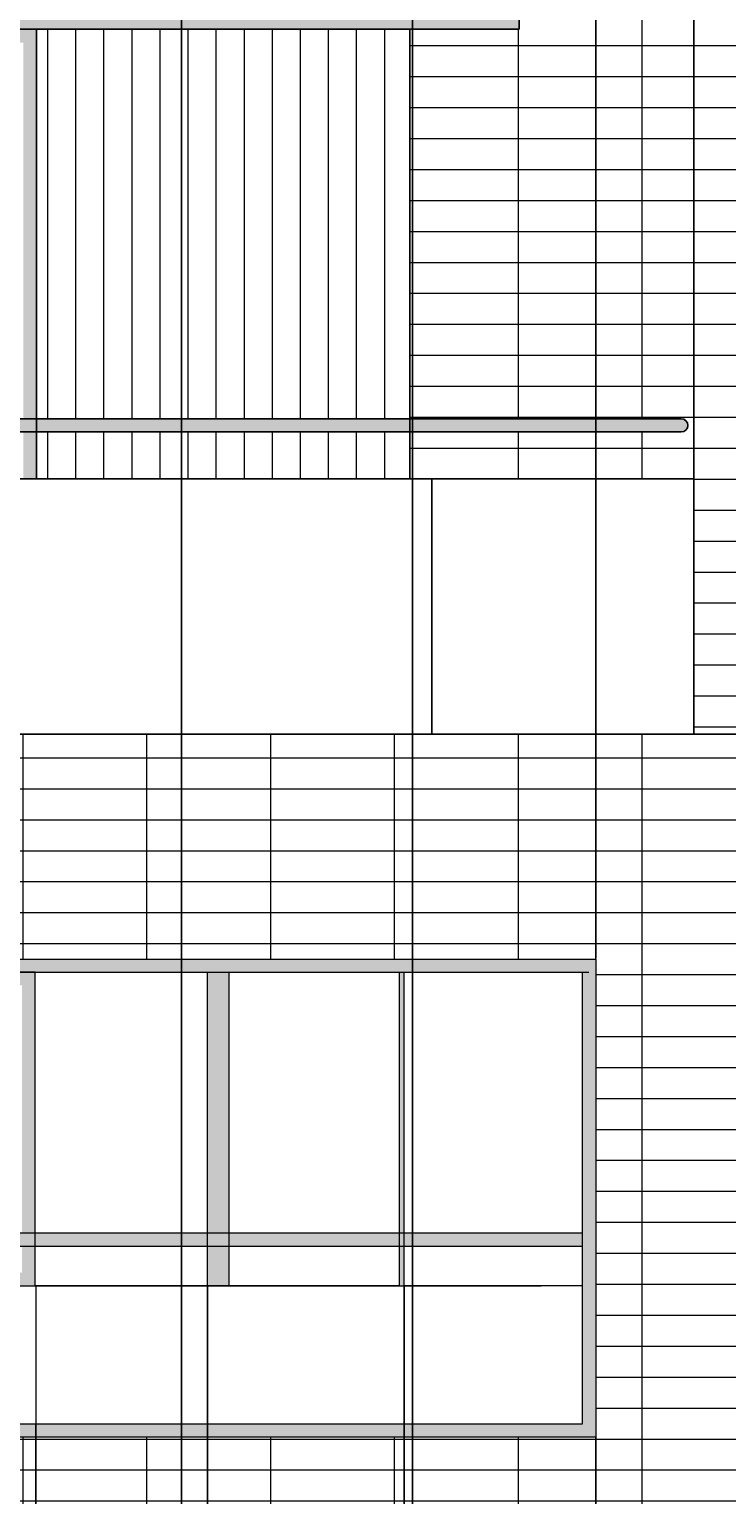
# Model space of a CAD drawing. Units: inches. Extents: x 241 to 943, y 109 to 1396.
# Tile 12 of 34: x 507 to 613, y 620 to 842. Entities that reach past the tile are written whole.
import ezdxf

# ---------------------------------------------------------------- set-up
doc = ezdxf.new("R2010")
doc.units = ezdxf.units.IN
doc.header["$MEASUREMENT"] = 0
for name, color, linetype, lineweight in [('A-ANNO-DIMS', 2, 'Continuous', 18), ('A-ELEV', 7, 'Continuous', 25), ('A-ELEV-SHAD', 9, 'Continuous', 13), ('A-GLAZ', 4, 'Continuous', 18), ('A-GLAZ-PATT', 18, 'Continuous', 13), ('A-WALL-PATT', 8, 'Continuous', 13)]:
    doc.layers.add(name, color=color, linetype=linetype, lineweight=lineweight)
doc.styles.get("Standard").update_dxf_attribs({"font": 'arial.ttf'})
doc.dimstyles.get("Standard").update_dxf_attribs({"dimtxt": 1.4375, "dimasz": 0.18, "dimexe": 0.18, "dimexo": 0.0625, "dimgap": 0.09, "dimtad": 0, "dimtih": 1, "dimtoh": 1, "dimdec": 4, "dimzin": 0, "dimdsep": 46, "dimlunit": 4, "dimtxsty": 'Standard', "dimcen": 0.09, "dimadec": 0, "dimazin": 0, "dimtfac": 1, "dimtdec": 4, "dimtofl": 0, "dimtmove": 0, "dimatfit": 3, "dimfxl": 1, "dimtolj": 1, "dimtzin": 0, "dimarcsym": 0})

# ---------------------------------------------------------------- blocks, each defined once
blk = doc.blocks.new('*D7')
at = {"layer": 'A-ANNO-DIMS', "color": 0, "lineweight": -2, "transparency": 16777216}
for p, q in [((508.24, 1336.12), (244.31, 1336.12)), ((244.49, 1335.94), (244.49, 753.25)), ((244.49, 168.92), (244.49, 751.6)), ((303.17, 168.74), (244.31, 168.74))]:
    blk.add_line(p, q, dxfattribs=at)
at = {"layer": 'A-ANNO-DIMS', "color": 0, "transparency": 16777216}
for points in [[(244.46, 1335.94), (244.52, 1335.94), (244.49, 1336.12)], [(244.46, 168.92), (244.52, 168.92), (244.49, 168.74)]]:
    blk.add_solid(points, dxfattribs=at)
at = {"layer": 'Defpoints', "color": 0, "transparency": 16777216}
for p in [(244.49, 1336.12), (508.31, 1336.12), (303.24, 168.74)]:
    blk.add_point(p, dxfattribs=at)
at = {"layer": 'A-ANNO-DIMS', "color": 0, "transparency": 16777216, "insert": (244.49, 752.43), "char_height": 1.438, "attachment_point": 5}
blk.add_mtext('\\A1;1167.4', dxfattribs=at)
blk = doc.blocks.new('*D11')
at = {"layer": 'A-ANNO-DIMS', "color": 0, "lineweight": -2, "transparency": 16777216}
for p, q in [((500.33, 384.24), (500.33, 1395.05)), ((500.51, 1394.87), (513.31, 1394.87)), ((530.05, 1394.87), (517.25, 1394.87)), ((530.23, 384.24), (530.23, 1395.05))]:
    blk.add_line(p, q, dxfattribs=at)
at = {"layer": 'A-ANNO-DIMS', "color": 0, "transparency": 16777216}
for points in [[(500.51, 1394.9), (500.51, 1394.84), (500.33, 1394.87)], [(530.05, 1394.9), (530.05, 1394.84), (530.23, 1394.87)]]:
    blk.add_solid(points, dxfattribs=at)
at = {"layer": 'Defpoints', "color": 0, "transparency": 16777216}
for p in [(530.23, 1394.87), (500.33, 384.18), (530.23, 384.18)]:
    blk.add_point(p, dxfattribs=at)
at = {"layer": 'A-ANNO-DIMS', "color": 0, "transparency": 16777216, "insert": (515.28, 1394.87), "char_height": 1.438, "attachment_point": 5}
blk.add_mtext('\\A1;29.9', dxfattribs=at)
blk = doc.blocks.new('*D12')
at = {"layer": 'A-ANNO-DIMS', "color": 0, "lineweight": -2, "transparency": 16777216}
for p, q in [((530.23, 384.24), (530.23, 1395.05)), ((530.41, 1394.87), (587.56, 1394.87)), ((650.73, 1394.87), (593.58, 1394.87)), ((650.91, 384.24), (650.91, 1395.05))]:
    blk.add_line(p, q, dxfattribs=at)
at = {"layer": 'A-ANNO-DIMS', "color": 0, "transparency": 16777216}
for points in [[(530.41, 1394.9), (530.41, 1394.84), (530.23, 1394.87)], [(650.73, 1394.9), (650.73, 1394.84), (650.91, 1394.87)]]:
    blk.add_solid(points, dxfattribs=at)
at = {"layer": 'Defpoints', "color": 0, "transparency": 16777216}
for p in [(650.91, 1394.87), (530.23, 384.18), (650.91, 384.18)]:
    blk.add_point(p, dxfattribs=at)
at = {"layer": 'A-ANNO-DIMS', "color": 0, "transparency": 16777216, "insert": (590.57, 1394.87), "char_height": 1.438, "attachment_point": 5}
blk.add_mtext('\\A1;120.68', dxfattribs=at)
blk = doc.blocks.new('*D62')
at = {"layer": 'A-ANNO-DIMS', "color": 0, "lineweight": -2, "transparency": 16777216}
for p, q in [((424.11, 568.89), (424.11, 1395.05)), ((424.29, 1394.87), (492.35, 1394.87)), ((565.02, 1394.87), (496.96, 1394.87)), ((565.2, 568.89), (565.2, 1395.05))]:
    blk.add_line(p, q, dxfattribs=at)
at = {"layer": 'A-ANNO-DIMS', "color": 0, "transparency": 16777216}
for points in [[(424.29, 1394.9), (424.29, 1394.84), (424.11, 1394.87)], [(565.02, 1394.9), (565.02, 1394.84), (565.2, 1394.87)]]:
    blk.add_solid(points, dxfattribs=at)
at = {"layer": 'Defpoints', "color": 0, "transparency": 16777216}
for p in [(565.2, 1394.87), (424.11, 568.83), (565.2, 568.83)]:
    blk.add_point(p, dxfattribs=at)
at = {"layer": 'A-ANNO-DIMS', "color": 0, "transparency": 16777216, "insert": (494.66, 1394.87), "char_height": 1.438, "attachment_point": 5}
blk.add_mtext('\\A1;141.1', dxfattribs=at)
blk = doc.blocks.new('*D65')
at = {"layer": 'A-ANNO-DIMS', "color": 0, "lineweight": -2, "transparency": 16777216}
for p, q in [((424.11, 700.85), (424.11, 1395.05)), ((424.29, 1394.87), (505.52, 1394.87)), ((592.77, 1394.87), (511.54, 1394.87)), ((592.95, 700.85), (592.95, 1395.05))]:
    blk.add_line(p, q, dxfattribs=at)
at = {"layer": 'A-ANNO-DIMS', "color": 0, "transparency": 16777216}
for points in [[(424.29, 1394.9), (424.29, 1394.84), (424.11, 1394.87)], [(592.77, 1394.9), (592.77, 1394.84), (592.95, 1394.87)]]:
    blk.add_solid(points, dxfattribs=at)
at = {"layer": 'Defpoints', "color": 0, "transparency": 16777216}
for p in [(592.95, 1394.87), (424.11, 700.79), (592.95, 700.79)]:
    blk.add_point(p, dxfattribs=at)
at = {"layer": 'A-ANNO-DIMS', "color": 0, "transparency": 16777216, "insert": (508.53, 1394.87), "char_height": 1.438, "attachment_point": 5}
blk.add_mtext('\\A1;168.85', dxfattribs=at)
blk = doc.blocks.new('*D67')
at = {"layer": 'A-ANNO-DIMS', "color": 0, "lineweight": -2, "transparency": 16777216}
for p, q in [((389.04, 773.55), (389.04, 1395.05)), ((389.22, 1394.87), (495.34, 1394.87)), ((607.64, 1394.87), (501.52, 1394.87)), ((607.82, 773.55), (607.82, 1395.05))]:
    blk.add_line(p, q, dxfattribs=at)
at = {"layer": 'A-ANNO-DIMS', "color": 0, "transparency": 16777216}
for points in [[(389.22, 1394.9), (389.22, 1394.84), (389.04, 1394.87)], [(607.64, 1394.9), (607.64, 1394.84), (607.82, 1394.87)]]:
    blk.add_solid(points, dxfattribs=at)
at = {"layer": 'Defpoints', "color": 0, "transparency": 16777216}
for p in [(607.82, 1394.87), (389.04, 773.49), (607.82, 773.49)]:
    blk.add_point(p, dxfattribs=at)
at = {"layer": 'A-ANNO-DIMS', "color": 0, "transparency": 16777216, "insert": (498.43, 1394.87), "char_height": 1.438, "attachment_point": 5}
blk.add_mtext('\\A1;218.77', dxfattribs=at)
blk = doc.blocks.new('*D82')
at = {"layer": 'A-ANNO-DIMS', "color": 0, "lineweight": -2, "transparency": 16777216}
for p, q in [((565.2, 568.89), (565.2, 1395.05)), ((565.38, 1394.87), (605.89, 1394.87)), ((651.42, 1394.87), (610.91, 1394.87)), ((651.6, 568.89), (651.6, 1395.05))]:
    blk.add_line(p, q, dxfattribs=at)
at = {"layer": 'A-ANNO-DIMS', "color": 0, "transparency": 16777216}
for points in [[(565.38, 1394.9), (565.38, 1394.84), (565.2, 1394.87)], [(651.42, 1394.9), (651.42, 1394.84), (651.6, 1394.87)]]:
    blk.add_solid(points, dxfattribs=at)
at = {"layer": 'Defpoints', "color": 0, "transparency": 16777216}
for p in [(651.6, 1394.87), (565.2, 568.83), (651.6, 568.83)]:
    blk.add_point(p, dxfattribs=at)
at = {"layer": 'A-ANNO-DIMS', "color": 0, "transparency": 16777216, "insert": (608.4, 1394.87), "char_height": 1.438, "attachment_point": 5}
blk.add_mtext('\\A1;86.40', dxfattribs=at)
blk = doc.blocks.new('*D83')
at = {"layer": 'A-ANNO-DIMS', "color": 0, "lineweight": -2, "transparency": 16777216}
for p, q in [((592.95, 700.85), (592.95, 1395.05)), ((593.13, 1394.87), (602.27, 1394.87)), ((617.58, 1394.87), (608.45, 1394.87)), ((617.76, 702.85), (617.76, 1395.05))]:
    blk.add_line(p, q, dxfattribs=at)
at = {"layer": 'A-ANNO-DIMS', "color": 0, "transparency": 16777216}
for points in [[(593.13, 1394.9), (593.13, 1394.84), (592.95, 1394.87)], [(617.58, 1394.9), (617.58, 1394.84), (617.76, 1394.87)]]:
    blk.add_solid(points, dxfattribs=at)
at = {"layer": 'Defpoints', "color": 0, "transparency": 16777216}
for p in [(617.76, 1394.87), (617.76, 702.79), (592.95, 700.79)]:
    blk.add_point(p, dxfattribs=at)
at = {"layer": 'A-ANNO-DIMS', "color": 0, "transparency": 16777216, "insert": (605.36, 1394.87), "char_height": 1.438, "attachment_point": 5}
blk.add_mtext('\\A1;24.805', dxfattribs=at)
blk = doc.blocks.new('*D99')
at = {"layer": 'A-ANNO-DIMS', "color": 0, "lineweight": -2, "transparency": 16777216}
for p, q in [((417.09, 181.71), (417.09, 1395.05)), ((417.27, 1394.87), (539.16, 1394.87)), ((667.21, 1394.87), (545.33, 1394.87)), ((667.39, 214.58), (667.39, 1395.05))]:
    blk.add_line(p, q, dxfattribs=at)
at = {"layer": 'A-ANNO-DIMS', "color": 0, "transparency": 16777216}
for points in [[(417.27, 1394.9), (417.27, 1394.84), (417.09, 1394.87)], [(667.21, 1394.9), (667.21, 1394.84), (667.39, 1394.87)]]:
    blk.add_solid(points, dxfattribs=at)
at = {"layer": 'Defpoints', "color": 0, "transparency": 16777216}
for p in [(667.39, 1394.87), (667.39, 214.52), (417.09, 181.65)]:
    blk.add_point(p, dxfattribs=at)
at = {"layer": 'A-ANNO-DIMS', "color": 0, "transparency": 16777216, "insert": (542.24, 1394.87), "char_height": 1.438, "attachment_point": 5}
blk.add_mtext('\\A1;250.30', dxfattribs=at)
blk = doc.blocks.new('*D127')
at = {"layer": 'A-ANNO-DIMS', "color": 0, "lineweight": -2, "transparency": 16777216}
for p, q in [((450.93, 651.27), (450.93, 109.81)), ((508.19, 630.34), (508.19, 109.81)), ((451.11, 109.99), (477.04, 109.99)), ((508.01, 109.99), (482.07, 109.99))]:
    blk.add_line(p, q, dxfattribs=at)
at = {"layer": 'A-ANNO-DIMS', "color": 0, "transparency": 16777216}
for points in [[(451.11, 110.02), (451.11, 109.96), (450.93, 109.99)], [(508.01, 110.02), (508.01, 109.96), (508.19, 109.99)]]:
    blk.add_solid(points, dxfattribs=at)
at = {"layer": 'Defpoints', "color": 0, "transparency": 16777216}
for p in [(450.93, 651.34), (508.19, 630.4), (508.19, 109.99)]:
    blk.add_point(p, dxfattribs=at)
at = {"layer": 'A-ANNO-DIMS', "color": 0, "transparency": 16777216, "insert": (479.56, 109.99), "char_height": 1.438, "attachment_point": 5}
blk.add_mtext('\\A1;57.26', dxfattribs=at)
blk = doc.blocks.new('*D128')
at = {"layer": 'A-ANNO-DIMS', "color": 0, "lineweight": -2, "transparency": 16777216}
for p, q in [((534.18, 651.27), (534.18, 109.81)), ((508.19, 630.34), (508.19, 109.81)), ((508.37, 109.99), (518.1, 109.99)), ((534, 109.99), (524.27, 109.99))]:
    blk.add_line(p, q, dxfattribs=at)
at = {"layer": 'A-ANNO-DIMS', "color": 0, "transparency": 16777216}
for points in [[(508.37, 110.02), (508.37, 109.96), (508.19, 109.99)], [(534, 110.02), (534, 109.96), (534.18, 109.99)]]:
    blk.add_solid(points, dxfattribs=at)
at = {"layer": 'Defpoints', "color": 0, "transparency": 16777216}
for p in [(534.18, 651.34), (508.19, 630.4), (534.18, 109.99)]:
    blk.add_point(p, dxfattribs=at)
at = {"layer": 'A-ANNO-DIMS', "color": 0, "transparency": 16777216, "insert": (521.18, 109.99), "char_height": 1.438, "attachment_point": 5}
blk.add_mtext('\\A1;25.987', dxfattribs=at)
blk = doc.blocks.new('*D129')
at = {"layer": 'A-ANNO-DIMS', "color": 0, "lineweight": -2, "transparency": 16777216}
for p, q in [((534.18, 651.27), (534.18, 109.81)), ((563.93, 651.27), (563.93, 109.81)), ((534.36, 109.99), (546.52, 109.99)), ((563.75, 109.99), (551.59, 109.99))]:
    blk.add_line(p, q, dxfattribs=at)
at = {"layer": 'A-ANNO-DIMS', "color": 0, "transparency": 16777216}
for points in [[(534.36, 110.02), (534.36, 109.96), (534.18, 109.99)], [(563.75, 110.02), (563.75, 109.96), (563.93, 109.99)]]:
    blk.add_solid(points, dxfattribs=at)
at = {"layer": 'Defpoints', "color": 0, "transparency": 16777216}
for p in [(534.18, 651.34), (563.93, 651.34), (563.93, 109.99)]:
    blk.add_point(p, dxfattribs=at)
at = {"layer": 'A-ANNO-DIMS', "color": 0, "transparency": 16777216, "insert": (549.05, 109.99), "char_height": 1.438, "attachment_point": 5}
blk.add_mtext('\\A1;29.75', dxfattribs=at)
blk = doc.blocks.new('*D130')
at = {"layer": 'A-ANNO-DIMS', "color": 0, "lineweight": -2, "transparency": 16777216}
for p, q in [((563.93, 651.27), (563.93, 109.81)), ((592.95, 628.34), (592.95, 109.81)), ((564.11, 109.99), (575.35, 109.99)), ((592.77, 109.99), (581.53, 109.99))]:
    blk.add_line(p, q, dxfattribs=at)
at = {"layer": 'A-ANNO-DIMS', "color": 0, "transparency": 16777216}
for points in [[(564.11, 110.02), (564.11, 109.96), (563.93, 109.99)], [(592.77, 110.02), (592.77, 109.96), (592.95, 109.99)]]:
    blk.add_solid(points, dxfattribs=at)
at = {"layer": 'Defpoints', "color": 0, "transparency": 16777216}
for p in [(563.93, 651.34), (592.95, 628.4), (592.95, 109.99)]:
    blk.add_point(p, dxfattribs=at)
at = {"layer": 'A-ANNO-DIMS', "color": 0, "transparency": 16777216, "insert": (578.44, 109.99), "char_height": 1.438, "attachment_point": 5}
blk.add_mtext('\\A1;29.025', dxfattribs=at)

msp = doc.modelspace()

# ---------------------------------------------------------------- hatches: boundary and pattern name
at = {"layer": 'A-ELEV-SHAD'}
h = msp.add_hatch(color=256, dxfattribs=at)
h.dxf.hatch_style = 1
h.paths.add_polyline_path([(508.3064, 1070.8538), (377.0391, 1070.8538), (377.0391, 1009.5382), (508.3064, 1009.5382)])
h.paths.add_polyline_path([(508.3064, 1238.8538), (377.0391, 1238.8538), (377.0391, 1177.5382), (508.3064, 1177.5382)])
h.paths.add_polyline_path([(581.3632, 902.8538), (568.1348, 902.8538), (553.5166, 902.8538), (377.0391, 902.8538), (377.0391, 841.5382), (553.5166, 841.5382), (564.8076, 841.5382), (581.3632, 841.5382)])
h.paths.add_polyline_path([(820.8374, 1275.9142), (747.7579, 1275.9142), (747.7579, 1238.8538), (820.8374, 1238.8538)])
h.paths.add_polyline_path([(820.8374, 1238.8538), (747.7579, 1238.8538), (747.9341, 1223.0633), (820.8374, 1223.0633)])
h.paths.add_polyline_path([(396.3125, 841.5382), (377.0391, 841.5382), (377.0391, 734.8538), (389.0429, 734.8538), (389.0429, 735.188), (389.0429, 773.4916), (396.3125, 773.4916), (396.3125, 780.5808), (390.5597, 780.5808), (388.0428, 780.5808, -1), (388.0428, 782.5808), (390.5597, 782.5808), (396.3125, 782.5808)])
h = msp.add_hatch(color=256, dxfattribs=at)
h.dxf.hatch_style = 1
h.paths.add_polyline_path([(537.4269, 698.7912), (534.1778, 698.7912), (534.1778, 659.3434), (537.4269, 659.3434)])
h.paths.add_polyline_path([(508.0803, 698.7912), (450.9259, 698.7912), (450.9259, 659.3434), (452.9259, 659.3434), (452.9259, 696.7912), (506.0803, 696.7912), (506.0803, 659.3434), (508.0803, 659.3434)])
h.paths.add_polyline_path([(481.5031, 696.7912), (479.5031, 696.7912), (479.5031, 659.3434), (481.5031, 659.3434)], flags=17)
h.paths.add_polyline_path([(481.5031, 657.3434), (479.5031, 657.3434), (479.5031, 653.3371), (481.5031, 653.3371)], flags=17)
h.paths.add_polyline_path([(508.0803, 657.3434), (506.0803, 657.3434), (506.0803, 653.3371), (452.9259, 653.3371), (452.9259, 657.3434), (450.9259, 657.3434), (450.9259, 651.3371), (508.0803, 651.3371)])
h.paths.add_polyline_path([(428.1173, 839.5382), (426.1173, 839.5382), (426.1173, 786.9154), (428.1173, 786.9154)], flags=17)
h.paths.add_polyline_path([(470.8692, 839.5382), (468.8692, 839.5382), (468.8692, 786.9154), (470.8692, 786.9154)], flags=17)
h.paths.add_polyline_path([(508.3064, 841.5382), (396.3125, 841.5382), (396.3125, 782.5808), (398.3125, 782.5808), (398.3125, 839.5382), (506.3064, 839.5382), (506.3064, 782.5808), (508.3064, 782.5808)])
h.paths.add_polyline_path([(398.3125, 780.5808), (396.3125, 780.5808), (396.3125, 773.4916), (398.3125, 773.4916)])
h.paths.add_polyline_path([(508.3064, 780.5808), (506.3064, 780.5808), (506.3064, 773.4916), (508.3064, 773.4916)])
h.paths.add_polyline_path([(715.6236, 841.5382), (678.2674, 841.5382), (678.2674, 734.8538), (715.6236, 734.8538)])
h.paths.add_polyline_path([(680.2674, 839.5382), (682.4526, 839.5382), (713.6236, 839.5382), (713.6236, 736.9235), (690.2047, 736.9235), (680.2674, 736.9235)], flags=16)
h.paths.add_polyline_path([(792.691, 841.5382), (747.7579, 841.5382), (747.7579, 734.8538), (754.5373, 734.8538), (754.5373, 736.9235), (754.5373, 839.5382), (756.7224, 839.5382), (787.8934, 839.5382), (787.8934, 765.9585), (792.691, 765.9585)])
h.paths.add_polyline_path([(659.2925, 1009.5382), (657.2925, 1009.5382), (657.2925, 902.8538), (659.2925, 902.8538)])
h.paths.add_polyline_path([(751.5078, 976.6275), (712.5839, 976.6275), (712.5839, 974.6275), (751.5078, 974.6275)])
h.paths.add_polyline_path([(470.8692, 1007.5382), (468.8692, 1007.5382), (468.8692, 954.9154), (470.8692, 954.9154)], flags=17)
h.paths.add_polyline_path([(508.3064, 1009.5382), (396.3125, 1009.5382), (396.3125, 950.5808), (398.3125, 950.5808), (398.3125, 1007.5382), (506.3064, 1007.5382), (506.3064, 950.5808), (508.3064, 950.5808)])
h.paths.add_polyline_path([(428.1173, 1007.5382), (426.1173, 1007.5382), (426.1173, 954.9154), (428.1173, 954.9154)], flags=17)
h.paths.add_polyline_path([(398.3125, 948.5808), (396.3125, 948.5808), (396.3125, 941.4916), (398.3125, 941.4916)])
h.paths.add_polyline_path([(508.3064, 948.5808), (506.3064, 948.5808), (506.3064, 941.4916), (508.3064, 941.4916)])
h.paths.add_polyline_path([(428.1173, 1175.5382), (426.1173, 1175.5382), (426.1173, 1122.9154), (428.1173, 1122.9154)], flags=17)
h.paths.add_polyline_path([(508.3064, 1177.5382), (396.3125, 1177.5382), (396.3125, 1118.5808), (398.3125, 1118.5808), (398.3125, 1175.5382), (506.3064, 1175.5382), (506.3064, 1118.5808), (506.8039, 1118.5808, -1), (506.8039, 1116.5808), (506.3064, 1116.5808), (506.3064, 1109.4916), (508.3064, 1109.4916)])
h.paths.add_polyline_path([(470.8692, 1175.5382), (468.8692, 1175.5382), (468.8692, 1122.9154), (470.8692, 1122.9154)], flags=17)
h.paths.add_polyline_path([(398.3125, 1116.5808), (396.3125, 1116.5808), (396.3125, 1109.4916), (398.3125, 1109.4916)], flags=17)
h.paths.add_polyline_path([(724.819, 1177.7336), (533.952, 1177.7336), (533.952, 1108.1686), (724.819, 1108.1686)])
h.paths.add_polyline_path([(535.952, 1175.7336), (722.819, 1175.7336), (722.819, 1110.1686), (535.952, 1110.1686)], flags=0)
h.paths.add_polyline_path([(622.521, 1136.0739), (643.4534, 1136.0739), (643.4534, 1134.0739), (622.521, 1134.0739)], flags=0)
h.paths.add_polyline_path([(722.819, 1175.7336), (535.952, 1175.7336), (535.952, 1110.1686), (722.819, 1110.1686)], flags=16)
h.paths.add_polyline_path([(565.947, 1151.5772), (535.952, 1151.5772), (535.952, 1149.5772), (565.947, 1149.5772)], flags=0)
h = msp.add_hatch(color=256, dxfattribs=at)
h.dxf.hatch_style = 1
h.paths.add_polyline_path([(537.4269, 657.3434), (534.1778, 657.3434), (534.1778, 651.3371), (537.4269, 651.3371)])
h.paths.add_polyline_path([(563.9297, 657.3434), (563.2023, 657.3434), (563.2023, 651.3371), (563.9297, 651.3371)])
h.paths.add_polyline_path([(563.9297, 698.7912), (563.2023, 698.7912), (563.2023, 659.3434), (563.9297, 659.3434)])
h.paths.add_polyline_path([(787.8934, 801.9791), (754.5373, 801.9791), (754.5373, 799.9791), (787.8934, 799.9791)])
h = msp.add_hatch(color=256, dxfattribs=at)
h.dxf.hatch_style = 1
h.paths.add_polyline_path([(537.4269, 566.8295), (534.1778, 566.8295), (534.1778, 527.3816), (537.4269, 527.3816)])
h.paths.add_polyline_path([(508.0803, 566.8295), (450.9259, 566.8295), (450.9259, 527.3816), (452.9259, 527.3816), (452.9259, 564.8295), (506.0803, 564.8295), (506.0803, 527.3816), (508.0803, 527.3816)])
h.paths.add_polyline_path([(481.5031, 564.8295), (479.5031, 564.8295), (479.5031, 527.3816), (481.5031, 527.3816)], flags=17)
h.paths.add_polyline_path([(481.5031, 525.3816), (479.5031, 525.3816), (479.5031, 521.3754), (481.5031, 521.3754)], flags=17)
h.paths.add_polyline_path([(508.0803, 525.3816), (506.0803, 525.3816), (506.0803, 521.3754), (452.9259, 521.3754), (452.9259, 525.3816), (450.9259, 525.3816), (450.9259, 519.3754), (508.0803, 519.3754)])
h.paths.add_polyline_path([(537.4269, 525.3816), (534.1778, 525.3816), (534.1778, 508.9074), (537.4269, 508.9074)])
h.paths.add_polyline_path([(749.6328, 702.7912), (617.7594, 702.7912), (617.7594, 700.7912), (747.6328, 700.7912), (747.6328, 628.4013), (617.7594, 628.4013), (617.7594, 626.4013), (749.6328, 626.4013)])
h.paths.add_polyline_path([(652.0129, 700.7912), (650.0129, 700.7912), (650.0129, 628.4013), (652.0129, 628.4013)], flags=17)
h.paths.add_polyline_path([(678.8698, 700.7912), (676.8698, 700.7912), (676.8698, 628.4013), (678.8698, 628.4013)], flags=17)
h.paths.add_polyline_path([(712.0171, 700.7912), (710.0171, 700.7912), (710.0171, 628.4013), (712.0171, 628.4013)], flags=17)
h.paths.add_polyline_path([(710.0171, 675.7856), (678.8698, 675.7856), (678.8698, 673.7856), (710.0171, 673.7856)], flags=17)
h.paths.add_polyline_path([(537.4269, 698.7912), (534.1778, 698.7912), (534.1778, 659.3434), (537.4269, 659.3434)], flags=0)
h.paths.add_polyline_path([(592.9542, 700.7912), (424.1086, 700.7912), (424.1086, 628.4013), (592.9542, 628.4013)])
h.paths.add_polyline_path([(590.8792, 698.7912), (590.8792, 630.4013), (426.1086, 630.4013), (426.1086, 698.7912)], flags=16)
h.paths.add_polyline_path([(563.2023, 698.7912), (563.2023, 659.3434), (563.9297, 659.3434), (563.9297, 651.3371), (508.1906, 651.3371), (508.0803, 651.3371), (450.9259, 651.3371), (428.0291, 651.3371), (428.0291, 698.7912), (451.9767, 698.7912), (508.0803, 698.7912), (537.4269, 698.7912)], flags=0)
h.paths.add_polyline_path([(506.0803, 696.7912), (506.0803, 653.3371), (452.9259, 653.3371), (452.9259, 657.3434), (445.5808, 657.3434, -1), (445.5808, 659.3434), (452.9259, 659.3434), (452.9259, 696.7912)], flags=0)
h.paths.add_polyline_path([(563.9297, 698.7912), (563.2023, 698.7912), (563.2023, 659.3434), (563.9297, 659.3434)], flags=0)
at = {"layer": 'A-GLAZ-PATT'}
h = msp.add_hatch(dxfattribs=at)
h.set_pattern_fill('ANSI31', color=256, scale=34, angle=45)
h.paths.add_polyline_path([(486.3418, 786.9154), (413.1187, 786.9154), (413.1187, 761.2284), (486.3418, 761.2284)])
h.paths.add_polyline_path([(486.3418, 954.9154), (413.1187, 954.9154), (413.1187, 929.2284), (486.3418, 929.2284)])
h.paths.add_polyline_path([(462.1074, 289.6933), (390.895, 289.6933), (390.895, 277.4626), (390.895, 274.3507), (462.1074, 274.3507), (462.1074, 277.4626)])
h.paths.add_polyline_path([(500.3323, 289.6933), (479.596, 289.6933), (479.596, 274.3507), (500.3323, 274.3507)])
h.paths.add_polyline_path([(450.9259, 566.8295), (426.1086, 566.8295), (426.1086, 498.4395), (446.4348, 498.4395), (446.4348, 519.3754), (450.9259, 519.3754), (450.9259, 525.3816), (445.5808, 525.3816, -1), (445.5808, 527.3816), (450.9259, 527.3816)])
h.paths.add_polyline_path([(563.2023, 508.9074), (534.1778, 508.9074), (508.1906, 508.9074), (508.1906, 498.4395), (563.2023, 498.4395)])
h.paths.add_polyline_path([(747.6328, 700.7912), (712.0171, 700.7912), (712.0171, 628.4013), (747.6328, 628.4013)])
h.paths.add_polyline_path([(446.4348, 643.7483), (426.1086, 643.7483), (426.1086, 630.4013), (446.4348, 630.4013)])
h.paths.add_polyline_path([(564.8076, 841.5382), (553.5166, 841.5382), (508.3064, 841.5382), (508.3064, 782.5808), (564.8076, 782.5808)])
h.paths.add_polyline_path([(564.8076, 780.5808), (508.3064, 780.5808), (508.3064, 773.4916), (564.8076, 773.4916)])
h.paths.add_polyline_path([(792.691, 762.5799), (759.6248, 762.5799), (759.6248, 736.9235), (759.6248, 734.8538), (792.691, 734.8538)])
h.paths.add_polyline_path([(564.8076, 1009.5382), (553.5166, 1009.5382), (508.3064, 1009.5382), (508.3064, 950.5808), (562.3033, 950.5808, -1), (562.3033, 948.5808), (508.3064, 948.5808), (508.3064, 941.4916), (564.8076, 941.4916)])
h.paths.add_polyline_path([(486.3418, 1122.9154), (413.1187, 1122.9154), (413.1187, 1097.2284), (486.3418, 1097.2284)])
h = msp.add_hatch(color=256, dxfattribs=at)
h.dxf.hatch_style = 1
h.paths.add_polyline_path([(396.3125, 1118.5808), (390.5597, 1118.5808), (388.0428, 1118.5808, 1), (388.0428, 1116.5808), (390.5597, 1116.5808), (396.3125, 1116.5808)])
h.paths.add_polyline_path([(398.3125, 1118.5808), (396.3125, 1118.5808), (396.3125, 1116.5808), (398.3125, 1116.5808)])
h.paths.add_polyline_path([(413.1187, 1118.5808), (398.3125, 1118.5808), (398.3125, 1116.5808), (413.1187, 1116.5808)])
h.paths.add_polyline_path([(506.3064, 1118.5808), (486.3418, 1118.5808), (486.3418, 1116.5808), (506.3064, 1116.5808)])
h.paths.add_polyline_path([(506.8039, 1118.5808), (506.3064, 1118.5808), (506.3064, 1116.5808), (506.8039, 1116.5808, 1)])
h.paths.add_polyline_path([(396.3125, 950.5808), (390.5597, 950.5808), (388.0428, 950.5808, 1), (388.0428, 948.5808), (390.5597, 948.5808), (396.3125, 948.5808)])
h.paths.add_polyline_path([(398.3125, 950.5808), (396.3125, 950.5808), (396.3125, 948.5808), (398.3125, 948.5808)])
h.paths.add_polyline_path([(413.1187, 950.5808), (398.3125, 950.5808), (398.3125, 948.5808), (413.1187, 948.5808)])
h.paths.add_polyline_path([(506.3064, 950.5808), (486.3418, 950.5808), (486.3418, 948.5808), (506.3064, 948.5808)])
h.paths.add_polyline_path([(508.3064, 950.5808), (506.3064, 950.5808), (506.3064, 948.5808), (508.3064, 948.5808)])
h.paths.add_polyline_path([(562.3033, 950.5808), (508.3064, 950.5808), (508.3064, 948.5808), (562.3033, 948.5808, 1)])
h.paths.add_polyline_path([(396.3125, 782.5808), (390.5597, 782.5808), (388.0428, 782.5808, 1), (388.0428, 780.5808), (390.5597, 780.5808), (396.3125, 780.5808)])
h.paths.add_polyline_path([(398.3125, 782.5808), (396.3125, 782.5808), (396.3125, 780.5808), (398.3125, 780.5808)])
h.paths.add_polyline_path([(413.1187, 782.5808), (398.3125, 782.5808), (398.3125, 780.5808), (413.1187, 780.5808)])
h.paths.add_polyline_path([(506.3064, 782.5808), (486.3418, 782.5808), (486.3418, 780.5808), (506.3064, 780.5808)])
h.paths.add_polyline_path([(508.3064, 782.5808), (506.3064, 782.5808), (506.3064, 780.5808), (508.3064, 780.5808)])
h.paths.add_polyline_path([(564.8076, 782.5808), (508.3064, 782.5808), (508.3064, 780.5808), (564.8076, 780.5808)])
h.paths.add_polyline_path([(605.9087, 782.5808), (564.8076, 782.5808), (564.8076, 780.5808), (605.9087, 780.5808, 1)])
h.paths.add_polyline_path([(450.9259, 659.3434), (445.5808, 659.3434, 1), (445.5808, 657.3434), (450.9259, 657.3434)])
h.paths.add_polyline_path([(452.9259, 659.3434), (450.9259, 659.3434), (450.9259, 657.3434), (452.9259, 657.3434)])
h.paths.add_polyline_path([(506.0803, 659.3434), (452.9259, 659.3434), (452.9259, 657.3434), (506.0803, 657.3434)])
h.paths.add_polyline_path([(508.0803, 659.3434), (506.0803, 659.3434), (506.0803, 657.3434), (508.0803, 657.3434)])
h.paths.add_polyline_path([(563.2023, 659.3434), (537.4269, 659.3434), (537.4269, 657.3434), (563.2023, 657.3434)])
h.paths.add_polyline_path([(590.8792, 659.3434), (563.9297, 659.3434), (563.9297, 657.3434), (590.8792, 657.3434)])
h.paths.add_polyline_path([(563.9297, 659.3434), (563.2023, 659.3434), (563.2023, 657.3434), (563.9297, 657.3434)])
h.paths.add_polyline_path([(537.4269, 659.3434), (534.1778, 659.3434), (534.1778, 657.3434), (537.4269, 657.3434)])
h.paths.add_polyline_path([(534.1778, 659.3434), (508.0803, 659.3434), (508.0803, 657.3434), (534.1778, 657.3434)])
h.paths.add_polyline_path([(450.9259, 527.3816), (445.5808, 527.3816, 1), (445.5808, 525.3816), (450.9259, 525.3816)])
h.paths.add_polyline_path([(452.9259, 527.3816), (450.9259, 527.3816), (450.9259, 525.3816), (452.9259, 525.3816)])
h.paths.add_polyline_path([(479.5031, 527.3816), (452.9259, 527.3816), (452.9259, 525.3816), (479.5031, 525.3816)])
h.paths.add_polyline_path([(481.5031, 527.3816), (479.5031, 527.3816), (479.5031, 525.3816), (481.5031, 525.3816)])
h.paths.add_polyline_path([(506.0803, 527.3816), (481.5031, 527.3816), (481.5031, 525.3816), (506.0803, 525.3816)])
h.paths.add_polyline_path([(508.0803, 527.3816), (506.0803, 527.3816), (506.0803, 525.3816), (508.0803, 525.3816)])
h.paths.add_polyline_path([(563.2023, 527.3816), (508.0803, 527.3816), (508.0803, 525.3816), (563.2023, 525.3816)])
at = {"layer": 'A-WALL-PATT'}
h = msp.add_hatch(dxfattribs=at)
h.set_pattern_fill('GRATE', color=256, scale=150)
h.paths.add_polyline_path([(747.7579, 1238.8538), (747.7579, 1275.9142), (747.7579, 1336.1154), (508.3064, 1336.1154), (508.3064, 1275.9142), (508.3064, 1238.8538), (508.3064, 1177.5382), (508.3064, 1109.4916), (508.3064, 1070.8538), (553.5166, 1070.8538), (749.6328, 1070.8538)])
h.paths.add_polyline_path([(533.952, 1108.1686), (533.952, 1177.7336), (533.952, 1303.0286), (724.819, 1303.0286), (724.819, 1108.1686)], flags=16)
h.paths.add_polyline_path([(535.952, 1110.1686), (535.952, 1175.7336), (722.819, 1175.7336), (722.819, 1110.1686)], flags=0)
h.paths.add_polyline_path([(643.4534, 1134.0739), (622.521, 1134.0739), (622.521, 1136.0739), (643.4534, 1136.0739)], flags=0)
h.paths.add_polyline_path([(617.7594, 568.8295), (617.7594, 734.8538), (377.0391, 734.8538), (377.0391, 566.8538), (377.0391, 400.8295), (417.0913, 400.8295), (618.9643, 400.8295)])
h.paths.add_polyline_path([(424.1086, 496.4395), (424.1086, 568.8295), (565.2023, 568.8295), (565.2023, 496.4395)], flags=16)
h.paths.add_polyline_path([(426.1086, 498.4395), (426.1086, 566.8295), (563.2023, 566.8295), (563.2023, 508.9074), (563.2023, 498.4395)], flags=0)
h.paths.add_polyline_path([(508.0803, 508.9074), (508.0803, 519.3754), (450.9259, 519.3754), (450.9259, 525.3816), (445.5808, 525.3816, -1), (445.5808, 527.3816), (450.9259, 527.3816), (450.9259, 566.8295), (508.0803, 566.8295), (537.4269, 566.8295), (537.4269, 508.9074)], flags=0)
h.paths.add_polyline_path([(506.0803, 521.3754), (452.9259, 521.3754), (452.9259, 564.8295), (506.0803, 564.8295)], flags=0)
h.paths.add_polyline_path([(424.1086, 628.4013), (424.1086, 700.7912), (592.9542, 700.7912), (592.9542, 628.4013)], flags=16)
h.paths.add_polyline_path([(426.1086, 630.4013), (426.1086, 698.7912), (590.8792, 698.7912), (590.8792, 630.4013)], flags=0)
h.paths.add_polyline_path([(508.1906, 651.3371), (508.0803, 651.3371), (450.9259, 651.3371), (428.0291, 651.3371), (428.0291, 698.7912), (451.9767, 698.7912), (508.0803, 698.7912), (537.4269, 698.7912), (563.2023, 698.7912), (563.2023, 659.3434), (563.9297, 659.3434), (563.9297, 651.3371)], flags=0)
h.paths.add_polyline_path([(506.0803, 653.3371), (452.9259, 653.3371), (452.9259, 657.3434), (445.5808, 657.3434, -1), (445.5808, 659.3434), (452.9259, 659.3434), (452.9259, 696.7912), (506.0803, 696.7912)], flags=0)
h = msp.add_hatch(dxfattribs=at)
h.set_pattern_fill('GRATE', color=256, scale=150)
h.paths.add_polyline_path([(820.8374, 1070.8538), (749.6328, 1070.8538), (553.5166, 1070.8538), (508.3064, 1070.8538), (508.3064, 1009.5382), (553.5166, 1009.5382), (564.8076, 1009.5382), (603.8694, 1009.5382), (751.5078, 1009.5382), (751.5078, 902.8538), (603.8694, 902.8538), (603.8694, 1009.5382), (564.8076, 1009.5382), (564.8076, 941.4916), (568.1348, 941.4916), (568.1348, 902.8538), (581.3632, 902.8538), (581.3632, 841.5382), (564.8076, 841.5382), (564.8076, 782.5808), (605.9087, 782.5808, -1), (605.9087, 780.5808), (564.8076, 780.5808), (564.8076, 773.4916), (597.514, 773.4916), (607.8162, 773.4916), (607.8162, 734.8538), (617.7594, 734.8538), (617.7594, 841.5382), (792.691, 841.5382), (792.691, 734.8538), (617.7594, 734.8538), (617.7594, 702.7912), (749.6328, 702.7912), (749.6328, 626.4013), (617.7594, 626.4013), (617.7594, 568.8295), (820.8374, 568.8295), (820.8374, 736.8295), (820.8374, 902.8538)])

# ---------------------------------------------------------------- linework, layer by layer
at = {"layer": 'A-ELEV'}
for p, q in [((581.3632, 841.5382), (581.3632, 902.8538)), ((377.0391, 841.5382), (553.5166, 841.5382)), ((508.3064, 841.5382), (508.3064, 773.4916)), ((553.5166, 841.5382), (564.8076, 841.5382)), ((564.8076, 841.5382), (564.8076, 773.4916)), ((564.8076, 841.5382), (581.3632, 841.5382)), ((486.3418, 782.5808), (605.9087, 782.5808)), ((486.3418, 780.5808), (605.9087, 780.5808)), ((597.514, 773.4916), (486.3418, 773.4916)), ((568.1348, 773.4916), (568.1348, 734.8538)), ((597.514, 773.4916), (607.8162, 773.4916)), ((607.8162, 734.8538), (607.8162, 773.4916)), ((377.0391, 734.8538), (792.691, 734.8538))]:
    msp.add_line(p, q, dxfattribs=at)
msp.add_arc((605.9087, 781.5808), 1, 270, 90, dxfattribs=at)
at = {"layer": 'A-GLAZ'}
for p, q in [((445.5808, 659.3434), (563.2023, 659.3434)), ((563.2023, 659.3434), (590.8792, 659.3434)), ((445.5808, 657.3434), (563.2023, 657.3434)), ((563.2023, 657.3434), (590.8792, 657.3434)), ((446.4348, 651.3371), (508.1906, 651.3371)), ((508.1906, 651.3371), (508.1906, 630.4013)), ((508.1906, 651.3371), (584.7135, 651.3371))]:
    msp.add_line(p, q, dxfattribs=at)
for points in [[(424.1086, 700.7912), (592.9542, 700.7912), (592.9542, 628.4013), (424.1086, 628.4013)], [(426.1086, 698.7912), (590.8792, 698.7912), (590.8792, 630.4013), (426.1086, 630.4013)], [(450.9259, 651.3371), (508.0803, 651.3371), (508.0803, 698.7912), (450.9259, 698.7912)], [(508.0803, 698.7912), (537.4269, 698.7912), (537.4269, 651.3371), (508.0803, 651.3371)], [(534.1778, 698.7912), (563.2023, 698.7912), (563.2023, 651.3371), (534.1778, 651.3371)]]:
    msp.add_lwpolyline(points, close=True, dxfattribs=at)
msp.add_lwpolyline([(590.8792, 651.3371), (563.9297, 651.3371), (563.9297, 698.7912), (591.9299, 698.7912)], dxfattribs=at)

# ---------------------------------------------------------------- dimensions: what is measured, and where the dimension line sits
at = {"layer": 'A-ANNO-DIMS'}
for base, p1, p2, override, picture, middle in [((607.8162, 1394.8654), (389.0429, 773.4916), (607.8162, 773.4916), {"dimdec": 2, "dimlfac": 1, "dimrnd": 0, "dimzin": 0, "dimdsep": 46, "dimlunit": 2}, '*D67', (498.4295, 1394.8654)), ((667.3935, 1394.8654), (417.0913, 181.649), (667.3935, 214.5189), {"dimdec": 2, "dimlfac": 1, "dimrnd": 0, "dimzin": 0, "dimdsep": 46, "dimlunit": 2}, '*D99', (542.2424, 1394.8654)), ((565.2023, 1394.8654), (424.1086, 568.8295), (565.2023, 568.8295), {"dimdec": 1, "dimlfac": 1, "dimrnd": 0, "dimzin": 0, "dimdsep": 46, "dimlunit": 2}, '*D62', (494.6554, 1394.8654)), ((592.9542, 1394.8654), (424.1086, 700.7912), (592.9542, 700.7912), {"dimdec": 2, "dimlfac": 1, "dimrnd": 0, "dimzin": 0, "dimdsep": 46, "dimlunit": 2}, '*D65', (508.5314, 1394.8654)), ((530.2303, 1394.8654), (500.3323, 384.1784), (530.2303, 384.1784), {"dimdec": 1, "dimlfac": 1, "dimrnd": 0, "dimzin": 0, "dimdsep": 46, "dimlunit": 2}, '*D11', (515.2813, 1394.8654)), ((650.907, 1394.8654), (530.2303, 384.1784), (650.907, 384.1784), {"dimdec": 2, "dimlfac": 1, "dimrnd": 0, "dimzin": 0, "dimdsep": 46, "dimlunit": 2}, '*D12', (590.5686, 1394.8654)), ((651.5974, 1394.8654), (565.2023, 568.8295), (651.5974, 568.8295), {"dimdec": 2, "dimlfac": 1, "dimrnd": 0, "dimzin": 0, "dimdsep": 46, "dimlunit": 2}, '*D82', (608.3998, 1394.8654)), ((617.7594, 1394.8654), (592.9542, 700.7912), (617.7594, 702.7912), {"dimdec": 3, "dimlfac": 1, "dimrnd": 0, "dimzin": 0, "dimdsep": 46, "dimlunit": 2}, '*D83', (605.3568, 1394.8654)), ((508.1906, 109.9907), (450.9259, 651.3371), (508.1906, 630.4013), {"dimdec": 2, "dimlfac": 1, "dimrnd": 0, "dimzin": 0, "dimdsep": 46, "dimlunit": 2}, '*D127', (479.5582, 109.9907)), ((534.1778, 109.9907), (508.1906, 630.4013), (534.1778, 651.3371), {"dimdec": 3, "dimlfac": 1, "dimrnd": 0, "dimzin": 0, "dimdsep": 46, "dimlunit": 2}, '*D128', (521.1842, 109.9907)), ((563.9297, 109.9907), (534.1778, 651.3371), (563.9297, 651.3371), {"dimdec": 2, "dimlfac": 1, "dimrnd": 0, "dimzin": 0, "dimdsep": 46, "dimlunit": 2}, '*D129', (549.0538, 109.9907)), ((592.954223, 109.990742), (563.92972, 651.337109), (592.954223, 628.401255), {"dimdec": 3, "dimlfac": 1, "dimrnd": 0, "dimzin": 0, "dimdsep": 46, "dimlunit": 2}, '*D130', (578.441971, 109.990742))]:
    dim = msp.add_linear_dim(base=base, p1=p1, p2=p2, dimstyle='Standard', override=override, dxfattribs=at)
    dim.commit()
    dim.dimension.update_dxf_attribs({"geometry": picture, "text_midpoint": middle})
dim = msp.add_linear_dim(base=(244.4858, 1336.1154), p1=(303.2358, 168.7407), p2=(508.3064, 1336.1154), angle=90, dimstyle='Standard', override={"dimdec": 1, "dimlfac": 1, "dimrnd": 0, "dimzin": 0, "dimdsep": 46, "dimlunit": 2}, dxfattribs=at)
dim.commit()
dim.dimension.update_dxf_attribs({"geometry": '*D7', "text_midpoint": (244.4858, 752.4281)})

doc.saveas('drawing.dxf')
